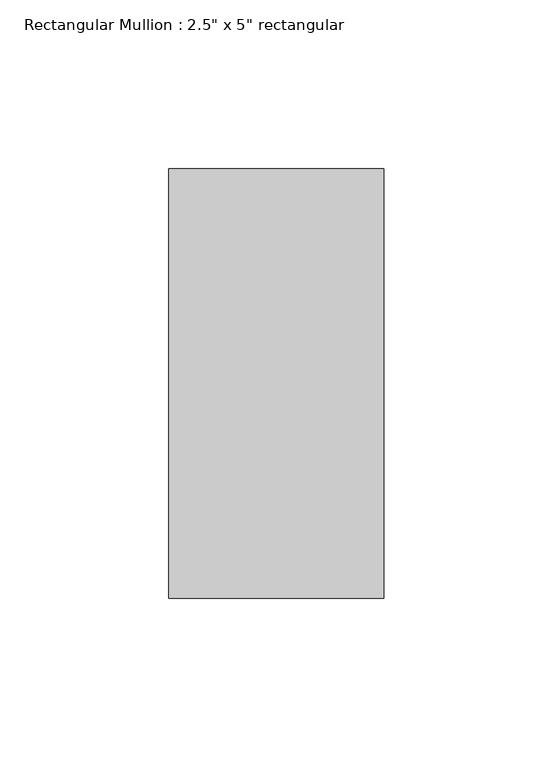
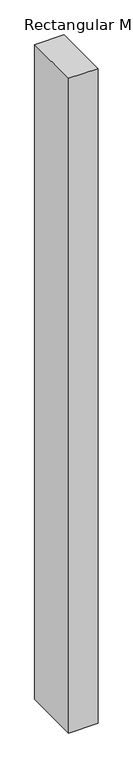
"""IFC4 building model written with IfcOpenShell, lengths in millimetres: member geometry."""

from ifc_helpers import new_model, si_unit, frame, origin, place, context, project, spatial, polyline, outline, extrude, source, transform, mapped, element, save


def member_fe23b6ba(model_context):
    return source(origin(), model_context, "Body", "SweptSolid", [
        extrude(outline(polyline([(31.75, 63.5), (31.75, -63.5), (-31.75, -63.5), (-31.75, 63.5), (31.75, 63.5)])), frame((0.0, 0.0, -1492.2228074), z_axis=(0.0, 0.0, 1.0), x_axis=(1.0, 0.0, 0.0)), (0.0, 0.0, 1.0), 1492.2228074),
    ])


if __name__ == "__main__":
    model = new_model("IFC4")
    model_context = context("Model", 3, world=origin())
    ifc_project = project(units=[si_unit("LENGTHUNIT", "METRE", prefix="MILLI")], contexts=[model_context])
    site = spatial("IfcSite", under=ifc_project)
    building = spatial("IfcBuilding", under=site)
    placement = place(None, origin())
    member_shape = member_fe23b6ba(model_context)
    element("IfcMember", 1, ObjectType="Rectangular Mullion : 2.5\" x 5\" rectangular", at=placement, inside=building, context=model_context, shape_type="MappedRepresentation", body=[
        mapped(member_shape, transform((0.0, 0.0, 0.0), x_axis=(1.0, 0.0, 0.0), y_axis=(0.0, 1.0, 0.0), z_axis=(0.0, 0.0, 1.0))),
    ])
    save(model, "model.ifc")

# Revit data of these elements
# Type "Rectangular Mullion : 2.5\" x 5\" rectangular"
#   built-in parameter 1007304 = 0.416667 (stored number, unit not read)
#   built-in parameter 1007301 = 0.104167 (stored number, unit not read)
#   built-in parameter 1007300 = 0.104167 (stored number, unit not read)
# Element 1 (IfcMember, "Rectangular Mullion : 2.5\" x 5\" rectangular")
#   Materials on its faces: "Aluminum"
# Materials
#   "Aluminum": class "Metal", colour RGB 247 247 247, transparency 0, Description = "Aluminum 6061", Cost = 0
